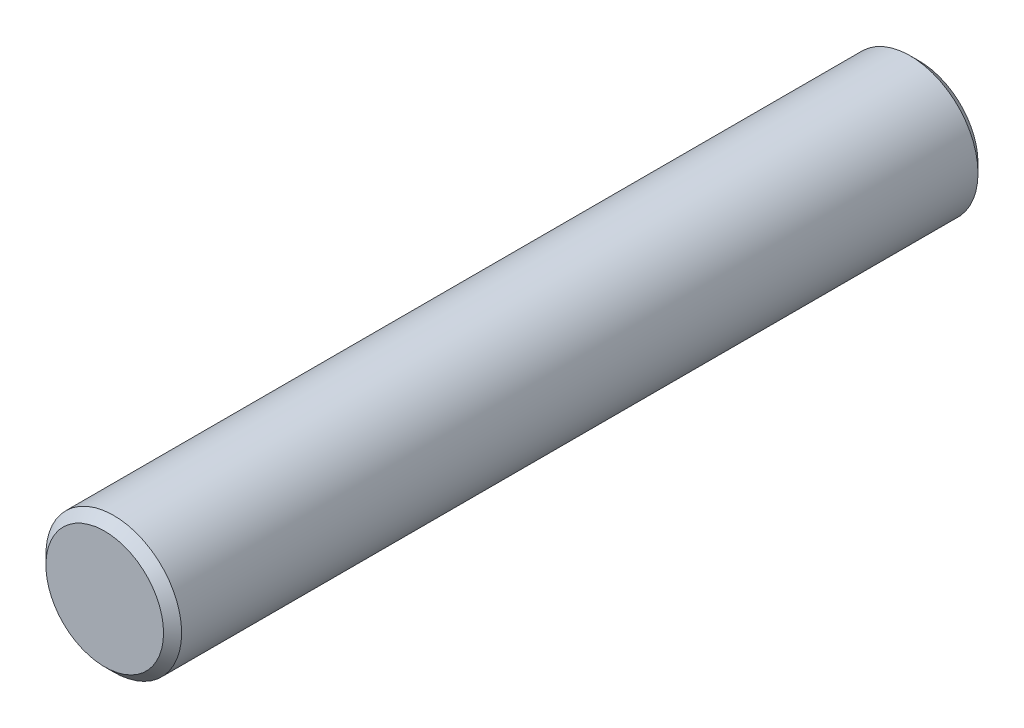
SolidWorks part; units mm, degrees
material "Plain Carbon Steel"
ref_plane "Front Plane" through (0, 0, 0) normal (0, 0, 1) x (1, 0, 0)
ref_plane "Top Plane" through (0, 0, 0) normal (0, 1, 0) x (1, 0, 0)
ref_plane "Right Plane" through (0, 0, 0) normal (1, 0, 0) x (0, 0, -1)
sketch "Pin Profile Ø3" plane through (0, 0, 0) normal (0, 0, 1) x (1, 0, 0)
  circle A0 centre (0, 0) radius 1.5
  dimension "D1" = 3
extrude "Pin Body Ø3x18" add sketch "Pin Profile Ø3" along normal mid plane 18
chamfer "End Chamfers 0.2x45°" distance 0.2 angle 45 2 edges at (1.5, 0, 9) (1.5, 0, -9)
